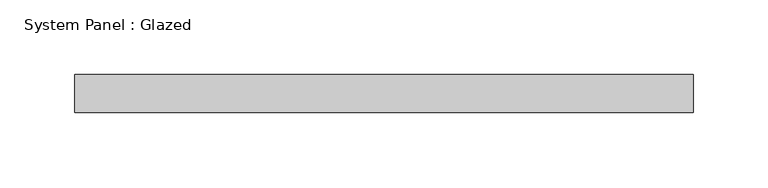
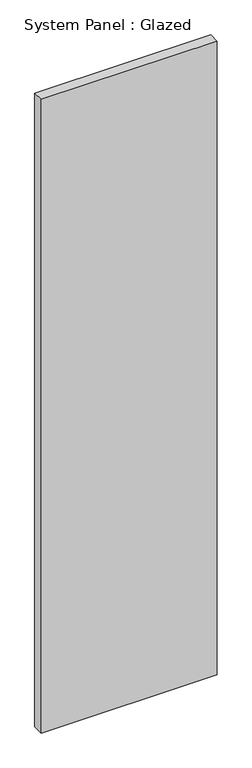
"""IFC4 building model written with IfcOpenShell, lengths in millimetres: plate geometry, System Panel : Glazed."""

from ifc_helpers import new_model, si_unit, origin, origin_with_axes, place, context, project, spatial, polyline, outline, extrude, source, transform, mapped, element, save


def system_panel_glazed_9aad7cd6(model_context):
    return source(origin(), model_context, "Body", "SweptSolid", [
        extrude(outline(polyline([(206.375, 19.05), (-206.375, 19.05), (-206.375, 44.45), (206.375, 44.45), (206.375, 19.05)])), origin_with_axes(), (0.0, 0.0, 1.0), 1569.2528693),
    ])


if __name__ == "__main__":
    model = new_model("IFC4")
    model_context = context("Model", 3, world=origin())
    ifc_project = project(units=[si_unit("LENGTHUNIT", "METRE", prefix="MILLI")], contexts=[model_context])
    site = spatial("IfcSite", under=ifc_project)
    building = spatial("IfcBuilding", under=site)
    placement = place(None, origin())
    system_panel_glazed_shape = system_panel_glazed_9aad7cd6(model_context)
    element("IfcPlate", 1, ObjectType="System Panel : Glazed", at=placement, inside=building, context=model_context, shape_type="MappedRepresentation", body=[
        mapped(system_panel_glazed_shape, transform((0.0, 0.0, 0.0), x_axis=(1.0, 0.0, 0.0), y_axis=(0.0, 1.0, 0.0), z_axis=(0.0, 0.0, 1.0))),
    ])
    save(model, "model.ifc")

# Revit data of these elements
# Type "System Panel : Glazed"
#   Construction Type Id = "GSP4R"
#   Analytic Construction = "1/8 in Pilkington single glazing"
#   Visual Light Transmittance = 0.9
#   Solar Heat Gain Coefficient = 0.86
#   Heat Transfer Coefficient (U) = 1.18115 BTU/(h·ft²·°F)
#   Define Thermal Properties by = 1
# Element 1 (IfcPlate, "System Panel : Glazed")
#   Materials on its faces: "Glass"
# Materials
#   "Glass": class "Glass", colour RGB 0 128 192, transparency 0.75, Description = "Soda Lime Glass", Cost = 0
